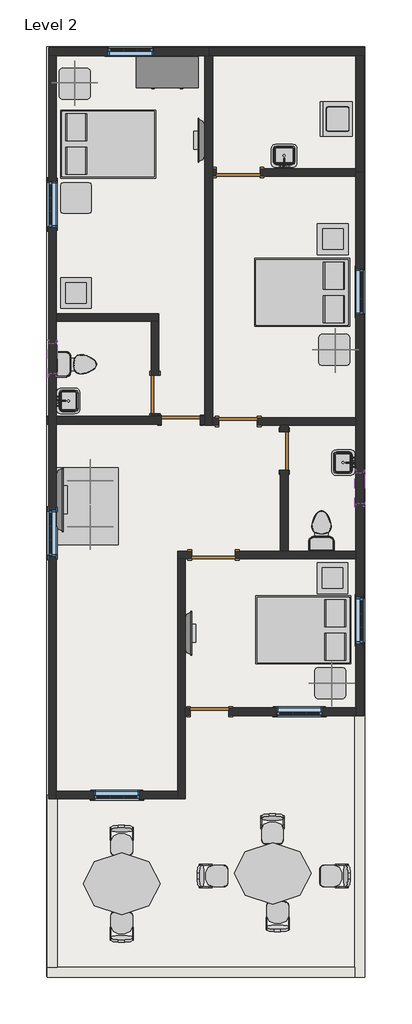
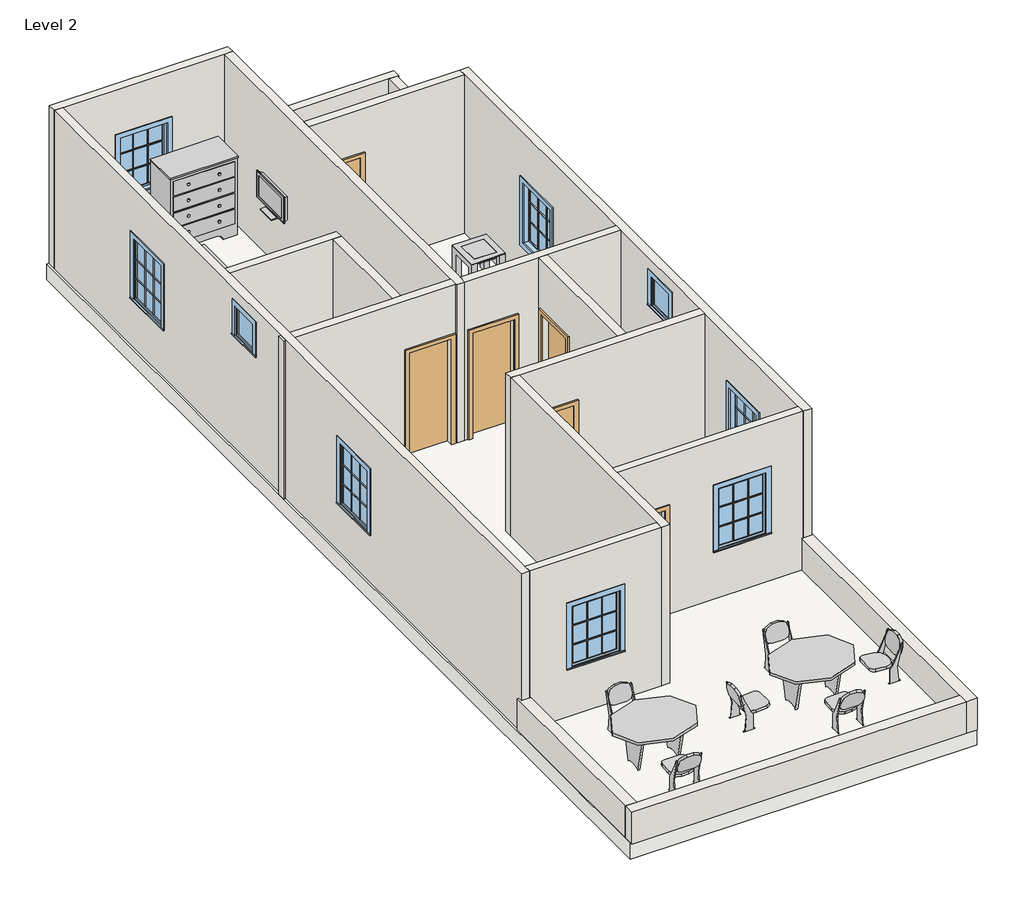
# One storey, incomplete: 23 furniture elements, 19 walls, 9 windows, 7 doors, 7 flow terminals, 5 geographic elements, 1 proxy, 1 slab.
"""IFC4 building model written with IfcOpenShell, lengths in millimetres."""

from ifc_helpers import new_model, si_unit, frame, origin, place, context, project, spatial, polyline, outline, extrude, faceted_brep, transform, mapped, element, save
from components import proxy_718fa39f, door_255cab33, door_059fdd7e, door_b6e9fca3, flow_terminal_accce45a, flow_terminal_62a433f7, toilet_domestic_3d_toilet_domestic_3d_f7549cf7, toilet_domestic_3d_toilet_domestic_3d_183bbd19, furniture_c8abb964, furniture_2babcf72, furniture_3d1d9cbc, furniture_56245f3a, furniture_fdf74506, furniture_b5c51a22, furniture_743965d2, furniture_31d08a24, furniture_e8434c74, rpc_plant_tropical_agave_1_5_93a2a214, window_5c190c7e, window_3d781103

model = new_model("IFC4")

# Units and contexts
model_context = context("Model", 3, world=origin())
ifc_project = project(units=[si_unit("LENGTHUNIT", "METRE", prefix="MILLI")], contexts=[model_context])

# Site, building, storey
site = spatial("IfcSite", under=ifc_project)
building = spatial("IfcBuilding", under=site)
storey = spatial("IfcBuildingStorey", under=building, Name="Level 2", Elevation=3048.0)

# Proxy
placement = place(None, origin())
proxy_shape = proxy_718fa39f(model_context)
element("IfcBuildingElementProxy", 1, Name="Washer : 27\" x 25\" x 35\"", ObjectType="Washer : 27\" x 25\" x 35\"", at=placement, inside=storey, context=model_context, shape_type="MappedRepresentation", body=[
    mapped(proxy_shape, transform((2989.1016011, 11111.8929316, 3048.0), x_axis=(0.0, 1.0000000000000007, 0.0), y_axis=(-1.0000000000000007, 0.0, 0.0), z_axis=(0.0, 0.0, 1.0))),
])

# Doors
door_shape = door_255cab33(model_context)
element("IfcDoor", 2, ObjectType="Single-Flush : 30\" x 80\"", at=placement, inside=storey, context=model_context, shape_type="MappedRepresentation", body=[
    mapped(door_shape, transform((-870.8676675, 6084.0104001, 3048.0), x_axis=(0.0, -1.0, 0.0), y_axis=(1.0, 0.0, 0.0), z_axis=(0.0, 0.0, 1.0))),
])
element("IfcDoor", 3, ObjectType="Single-Flush : 30\" x 80\"", at=placement, inside=storey, context=model_context, shape_type="MappedRepresentation", body=[
    mapped(door_shape, transform((773.4921844, 5550.6104001, 3048.0), x_axis=(-1.0, 0.0, 0.0), y_axis=(0.0, -1.0, 0.0), z_axis=(0.0, 0.0, 1.0))),
])
element("IfcDoor", 4, ObjectType="Single-Flush : 30\" x 80\"", at=placement, inside=storey, context=model_context, shape_type="MappedRepresentation", body=[
    mapped(door_shape, transform((1684.5721104, 4966.4104001, 3048.0), x_axis=(0.0, 1.0, 0.0), y_axis=(-1.0, 0.0, 0.0), z_axis=(0.0, 0.0, 1.0))),
])
element("IfcDoor", 5, ObjectType="Single-Flush : 30\" x 80\"", at=placement, inside=storey, context=model_context, shape_type="MappedRepresentation", body=[
    mapped(door_shape, transform((208.0520363, -189.7895999, 3048.0), x_axis=(-1.0, 0.0, 0.0), y_axis=(0.0, -1.0, 0.0), z_axis=(0.0, 0.0, 1.0))),
])
door_2_shape = door_059fdd7e(model_context)
element("IfcDoor", 6, ObjectType="Single-Flush : 30\" x 80\"", at=placement, inside=storey, context=model_context, shape_type="MappedRepresentation", body=[
    mapped(door_2_shape, transform((-362.8676675, 5576.0104001, 3048.0), x_axis=(1.0, 0.0, 0.0), y_axis=(0.0, 1.0, 0.0), z_axis=(0.0, 0.0, 1.0))),
])
door_3_shape = door_b6e9fca3(model_context)
element("IfcDoor", 7, ObjectType="Single-Flush : 34\" x 84\"", at=placement, inside=storey, context=model_context, shape_type="MappedRepresentation", body=[
    mapped(door_3_shape, transform((773.4921844, 10478.2104001, 3048.0), x_axis=(-1.0, 0.0, 0.0), y_axis=(0.0, -1.0, 0.0), z_axis=(0.0, 0.0, 1.0))),
])
element("IfcDoor", 8, ObjectType="Single-Flush : 34\" x 84\"", at=placement, inside=storey, context=model_context, shape_type="MappedRepresentation", body=[
    mapped(door_3_shape, transform((284.2520363, 2909.0104001, 3048.0), x_axis=(-1.0, 0.0, 0.0), y_axis=(0.0, -1.0, 0.0), z_axis=(0.0, 0.0, 1.0))),
])

# Flow terminals
flow_terminal_shape = flow_terminal_accce45a(model_context)
element("IfcFlowTerminal", 9, ObjectType="Floor Drain - Round : 5\" Strainer - 2\" Drain", at=placement, inside=storey, context=model_context, shape_type="MappedRepresentation", body=[
    mapped(flow_terminal_shape, transform((2849.6520363, 3798.0104001, 3048.0), x_axis=(1.0, 0.0, 0.0), y_axis=(0.0, 1.0, 0.0), z_axis=(0.0, 0.0, 1.0))),
])
element("IfcFlowTerminal", 10, ObjectType="Floor Drain - Round : 5\" Strainer - 2\" Drain", at=placement, inside=storey, context=model_context, shape_type="MappedRepresentation", body=[
    mapped(flow_terminal_shape, transform((-2331.9479637, 7125.4104001, 3048.0), x_axis=(1.0, 0.0, 0.0), y_axis=(0.0, 1.0, 0.0), z_axis=(0.0, 0.0, 1.0))),
])
flow_terminal_2_shape = flow_terminal_62a433f7(model_context)
element("IfcFlowTerminal", 11, ObjectType="Sink Vanity-Square : 20\" x 18\"", at=placement, inside=storey, context=model_context, shape_type="MappedRepresentation", body=[
    mapped(flow_terminal_2_shape, transform((-2634.4025626, 5941.3211595, 3048.0), x_axis=(0.0, 1.0000000000000002, 0.0), y_axis=(-1.0000000000000002, 0.0, 0.0), z_axis=(0.0, 0.0, 1.0))),
])
element("IfcFlowTerminal", 12, ObjectType="Sink Vanity-Square : 20\" x 18\"", at=placement, inside=storey, context=model_context, shape_type="MappedRepresentation", body=[
    mapped(flow_terminal_2_shape, transform((2898.1066352, 4753.4996407, 3048.0), x_axis=(0.0, -1.0, 0.0), y_axis=(1.0, 0.0, 0.0), z_axis=(0.0, 0.0, 1.0))),
])
element("IfcFlowTerminal", 13, ObjectType="Sink Vanity-Square : 20\" x 18\"", at=placement, inside=storey, context=model_context, shape_type="MappedRepresentation", body=[
    mapped(flow_terminal_2_shape, transform((1696.9412769, 10759.9558012, 3048.0), x_axis=(-1.0000000000000004, 0.0, 0.0), y_axis=(0.0, -1.0000000000000004, 0.0), z_axis=(0.0, 0.0, 1.0))),
])
toilet_domestic_3d_toilet_domestic_3d_shape = toilet_domestic_3d_toilet_domestic_3d_f7549cf7(model_context)
toilet_domestic_3d_toilet_domestic_3d_2_shape = toilet_domestic_3d_toilet_domestic_3d_183bbd19(model_context)
element("IfcFlowTerminal", 14, ObjectType="Toilet-Domestic-3D : Toilet-Domestic-3D", at=placement, inside=storey, context=model_context, shape_type="MappedRepresentation", body=[
    mapped(toilet_domestic_3d_toilet_domestic_3d_shape, transform((-2331.9716402, 6680.9104001, 3048.0), x_axis=(0.0, 1.0000000000000002, 0.0), y_axis=(-1.0000000000000002, 0.0, 0.0), z_axis=(0.0, 0.0, 1.0))),
    mapped(toilet_domestic_3d_toilet_domestic_3d_2_shape, transform((-2331.9716402, 6680.9104001, 3048.0), x_axis=(0.0, 1.0000000000000002, 0.0), y_axis=(-1.0000000000000002, 0.0, 0.0), z_axis=(0.0, 0.0, 1.0))),
])
element("IfcFlowTerminal", 15, ObjectType="Toilet-Domestic-3D : Toilet-Domestic-3D", at=placement, inside=storey, context=model_context, shape_type="MappedRepresentation", body=[
    mapped(toilet_domestic_3d_toilet_domestic_3d_shape, transform((2421.1721104, 3479.9064275, 3048.0), x_axis=(-1.0000000000000004, 0.0, 0.0), y_axis=(0.0, -1.0000000000000004, 0.0), z_axis=(0.0, 0.0, 1.0))),
    mapped(toilet_domestic_3d_toilet_domestic_3d_2_shape, transform((2421.1721104, 3479.9064275, 3048.0), x_axis=(-1.0000000000000004, 0.0, 0.0), y_axis=(0.0, -1.0000000000000004, 0.0), z_axis=(0.0, 0.0, 1.0))),
])

# Furniture
furniture_shape = furniture_c8abb964(model_context)
element("IfcFurniture", 16, ObjectType="Bed-Box : Double 53\" x 74\"", at=placement, inside=storey, context=model_context, shape_type="MappedRepresentation", body=[
    mapped(furniture_shape, transform((-2032.9774719, 10697.8579411, 3048.0), x_axis=(0.0, 1.0, 0.0), y_axis=(-1.0, 0.0, 0.0), z_axis=(0.0, 0.0, 1.0))),
])
element("IfcFurniture", 17, ObjectType="Bed-Box : Double 53\" x 74\"", at=placement, inside=storey, context=model_context, shape_type="MappedRepresentation", body=[
    mapped(furniture_shape, transform((2271.2815445, 8442.4628591, 3048.0), x_axis=(0.0, -1.0, 0.0), y_axis=(1.0, 0.0, 0.0), z_axis=(0.0, 0.0, 1.0))),
])
element("IfcFurniture", 18, ObjectType="Bed-Box : Double 53\" x 74\"", at=placement, inside=storey, context=model_context, shape_type="MappedRepresentation", body=[
    mapped(furniture_shape, transform((2296.6815445, 1765.7892779, 3048.0), x_axis=(0.0, -1.0000000000000002, 0.0), y_axis=(1.0000000000000002, 0.0, 0.0), z_axis=(0.0, 0.0, 1.0))),
])
furniture_2_shape = furniture_2babcf72(model_context)
element("IfcFurniture", 19, ObjectType="Dresser : 48\" x 60\" x 24\"", at=placement, inside=storey, context=model_context, shape_type="MappedRepresentation", body=[
    mapped(furniture_2_shape, transform((-360.9547039, 12822.5733542, 3048.0), x_axis=(1.0, 0.0, 0.0), y_axis=(0.0, 1.0, 0.0), z_axis=(0.0, 0.0, 1.0))),
])
furniture_3_shape = furniture_3d1d9cbc(model_context)
element("IfcFurniture", 20, ObjectType="Seating-Auditorium : 18\" x 24\" x 30\"", at=placement, inside=storey, context=model_context, shape_type="MappedRepresentation", body=[
    mapped(furniture_3_shape, transform((-1371.1200948, -2539.9141901, 3048.0), x_axis=(-1.0000000000000004, 0.0, 0.0), y_axis=(0.0, -1.0000000000000004, 0.0), z_axis=(0.0, 0.0, 1.0))),
])
element("IfcFurniture", 21, ObjectType="Seating-Auditorium : 18\" x 24\" x 30\"", at=placement, inside=storey, context=model_context, shape_type="MappedRepresentation", body=[
    mapped(furniture_3_shape, transform((1613.3799052, -2311.3141901, 3048.0), x_axis=(-1.0000000000000004, 0.0, 0.0), y_axis=(0.0, -1.0000000000000004, 0.0), z_axis=(0.0, 0.0, 1.0))),
])
element("IfcFurniture", 22, ObjectType="Seating-Auditorium : 18\" x 24\" x 30\"", at=placement, inside=storey, context=model_context, shape_type="MappedRepresentation", body=[
    mapped(furniture_3_shape, transform((1393.5241675, -4443.6650097, 3048.0), x_axis=(1.0, 0.0, 0.0), y_axis=(0.0, 1.0, 0.0), z_axis=(0.0, 0.0, 1.0))),
])
element("IfcFurniture", 23, ObjectType="Seating-Auditorium : 18\" x 24\" x 30\"", at=placement, inside=storey, context=model_context, shape_type="MappedRepresentation", body=[
    mapped(furniture_3_shape, transform((68.9766265, -3280.261731, 3048.0), x_axis=(0.0, -1.0000000000000007, 0.0), y_axis=(1.0000000000000007, 0.0, 0.0), z_axis=(0.0, 0.0, 1.0))),
])
element("IfcFurniture", 24, ObjectType="Seating-Auditorium : 18\" x 24\" x 30\"", at=placement, inside=storey, context=model_context, shape_type="MappedRepresentation", body=[
    mapped(furniture_3_shape, transform((2887.1274461, -3601.7174688, 3048.0), x_axis=(0.0, 1.000000000000001, 0.0), y_axis=(-1.000000000000001, 0.0, 0.0), z_axis=(0.0, 0.0, 1.0))),
])
element("IfcFurniture", 25, ObjectType="Seating-Auditorium : 18\" x 24\" x 30\"", at=placement, inside=storey, context=model_context, shape_type="MappedRepresentation", body=[
    mapped(furniture_3_shape, transform((-1692.5758325, -4646.8650097, 3048.0), x_axis=(1.0, 0.0, 0.0), y_axis=(0.0, 1.0, 0.0), z_axis=(0.0, 0.0, 1.0))),
])
furniture_4_shape = furniture_56245f3a(model_context)
element("IfcFurniture", 26, ObjectType="TV - Flat Screen : 32\"", at=placement, inside=storey, context=model_context, shape_type="MappedRepresentation", body=[
    mapped(furniture_4_shape, transform((47.9134127, 11109.265886, 4089.4), x_axis=(0.0, -1.0000000000000002, 0.0), y_axis=(1.0000000000000002, 0.0, 0.0), z_axis=(0.0, 0.0, 1.0))),
])
element("IfcFurniture", 27, ObjectType="TV - Flat Screen : 32\"", at=placement, inside=storey, context=model_context, shape_type="MappedRepresentation", body=[
    mapped(furniture_4_shape, transform((-216.00934, 1363.5549142, 3962.4), x_axis=(0.0, 1.0000000000000002, 0.0), y_axis=(-1.0000000000000002, 0.0, 0.0), z_axis=(0.0, 0.0, 1.0))),
])
furniture_5_shape = furniture_fdf74506(model_context)
element("IfcFurniture", 28, ObjectType="TV - Flat Screen : 50\"", at=placement, inside=storey, context=model_context, shape_type="MappedRepresentation", body=[
    mapped(furniture_5_shape, transform((-2756.00934, 4005.1549142, 4089.4), x_axis=(0.0, 1.0000000000000002, 0.0), y_axis=(-1.0000000000000002, 0.0, 0.0), z_axis=(0.0, 0.0, 1.0))),
])
furniture_6_shape = furniture_b5c51a22(model_context)
element("IfcFurniture", 29, ObjectType="Table-Coffee : 24\" x 24\" x 24\"", at=placement, inside=storey, context=model_context, shape_type="MappedRepresentation", body=[
    mapped(furniture_6_shape, transform((-2451.8137304, 7995.3993223, 3048.0), x_axis=(1.0, 0.0, 0.0), y_axis=(0.0, 1.0, 0.0), z_axis=(0.0, 0.0, 1.0))),
])
element("IfcFurniture", 30, ObjectType="Table-Coffee : 24\" x 24\" x 24\"", at=placement, inside=storey, context=model_context, shape_type="MappedRepresentation", body=[
    mapped(furniture_6_shape, transform((2628.1862696, 9062.1993223, 3048.0), x_axis=(1.0, 0.0, 0.0), y_axis=(0.0, 1.0, 0.0), z_axis=(0.0, 0.0, 1.0))),
])
element("IfcFurniture", 31, ObjectType="Table-Coffee : 24\" x 24\" x 24\"", at=placement, inside=storey, context=model_context, shape_type="MappedRepresentation", body=[
    mapped(furniture_6_shape, transform((2621.8362696, 2356.5993223, 3048.0), x_axis=(1.0, 0.0, 0.0), y_axis=(0.0, 1.0, 0.0), z_axis=(0.0, 0.0, 1.0))),
])
furniture_7_shape = furniture_743965d2(model_context)
element("IfcFurniture", 32, ObjectType="Table-Ellipse : 60\" x 48\"", at=placement, inside=storey, context=model_context, shape_type="MappedRepresentation", body=[
    mapped(furniture_7_shape, transform((-1531.8479637, -3593.3895999, 3048.0), x_axis=(1.0, 0.0, 0.0), y_axis=(0.0, 1.0, 0.0), z_axis=(0.0, 0.0, 1.0))),
])
element("IfcFurniture", 33, ObjectType="Table-Ellipse : 60\" x 48\"", at=placement, inside=storey, context=model_context, shape_type="MappedRepresentation", body=[
    mapped(furniture_7_shape, transform((1452.6520363, -3390.1895999, 3048.0), x_axis=(1.0, 0.0, 0.0), y_axis=(0.0, 1.0, 0.0), z_axis=(0.0, 0.0, 1.0))),
])
furniture_8_shape = furniture_31d08a24(model_context)
element("IfcFurniture", 34, ObjectType="Table-End : 24\" x 24\"", at=placement, inside=storey, context=model_context, shape_type="MappedRepresentation", body=[
    mapped(furniture_8_shape, transform((-2767.481594, 12078.4104001, 3048.0), x_axis=(1.0, 0.0, 0.0), y_axis=(0.0, 1.0, 0.0), z_axis=(0.0, 0.0, 1.0))),
])
element("IfcFurniture", 35, ObjectType="Table-End : 24\" x 24\"", at=placement, inside=storey, context=model_context, shape_type="MappedRepresentation", body=[
    mapped(furniture_8_shape, transform((-2742.081594, 9817.8104001, 3048.0), x_axis=(1.0, 0.0, 0.0), y_axis=(0.0, 1.0, 0.0), z_axis=(0.0, 0.0, 1.0))),
])
element("IfcFurniture", 36, ObjectType="Table-End : 24\" x 24\"", at=placement, inside=storey, context=model_context, shape_type="MappedRepresentation", body=[
    mapped(furniture_8_shape, transform((2363.318406, 6814.2604001, 3048.0), x_axis=(1.0, 0.0, 0.0), y_axis=(0.0, 1.0, 0.0), z_axis=(0.0, 0.0, 1.0))),
])
element("IfcFurniture", 37, ObjectType="Table-End : 24\" x 24\"", at=placement, inside=storey, context=model_context, shape_type="MappedRepresentation", body=[
    mapped(furniture_8_shape, transform((2287.118406, 222.9604001, 3048.0), x_axis=(1.0, 0.0, 0.0), y_axis=(0.0, 1.0, 0.0), z_axis=(0.0, 0.0, 1.0))),
])
furniture_9_shape = furniture_e8434c74(model_context)
element("IfcFurniture", 38, ObjectType="Table-Rectangular : 60\" x 48\"", at=placement, inside=storey, context=model_context, shape_type="MappedRepresentation", body=[
    mapped(furniture_9_shape, transform((-2204.9479637, 3874.2104001, 3048.0), x_axis=(0.0, 1.0, 0.0), y_axis=(-1.0, 0.0, 0.0), z_axis=(0.0, 0.0, 1.0))),
])

# Geographic elements
rpc_plant_tropical_agave_1_5_shape = rpc_plant_tropical_agave_1_5_93a2a214(model_context)
element("IfcGeographicElement", 39, ObjectType="RPC Plant - Tropical : Agave - 1.5'", at=placement, inside=storey, context=model_context, shape_type="MappedRepresentation", body=[
    mapped(rpc_plant_tropical_agave_1_5_shape, transform((-2458.9479637, 12256.2104001, 3657.6), x_axis=(1.0, 0.0, 0.0), y_axis=(0.0, 1.0, 0.0), z_axis=(0.0, 0.0, 1.0))),
])
element("IfcGeographicElement", 40, ObjectType="RPC Plant - Tropical : Agave - 1.5'", at=placement, inside=storey, context=model_context, shape_type="MappedRepresentation", body=[
    mapped(rpc_plant_tropical_agave_1_5_shape, transform((2697.2520363, 6966.6604001, 3657.6), x_axis=(1.0, 0.0, 0.0), y_axis=(0.0, 1.0, 0.0), z_axis=(0.0, 0.0, 1.0))),
])
element("IfcGeographicElement", 41, ObjectType="RPC Plant - Tropical : Agave - 1.5'", at=placement, inside=storey, context=model_context, shape_type="MappedRepresentation", body=[
    mapped(rpc_plant_tropical_agave_1_5_shape, transform((2621.0520363, 375.3604001, 3657.6), x_axis=(1.0, 0.0, 0.0), y_axis=(0.0, 1.0, 0.0), z_axis=(0.0, 0.0, 1.0))),
])
element("IfcGeographicElement", 42, ObjectType="RPC Plant - Tropical : Agave - 1.5'", at=placement, inside=storey, context=model_context, shape_type="MappedRepresentation", body=[
    mapped(rpc_plant_tropical_agave_1_5_shape, transform((-2154.1479637, 4382.2104001, 3708.4), x_axis=(1.0, 0.0, 0.0), y_axis=(0.0, 1.0, 0.0), z_axis=(0.0, 0.0, 1.0))),
])
element("IfcGeographicElement", 43, ObjectType="RPC Plant - Tropical : Agave - 1.5'", at=placement, inside=storey, context=model_context, shape_type="MappedRepresentation", body=[
    mapped(rpc_plant_tropical_agave_1_5_shape, transform((-2154.1479637, 3467.8104001, 3708.4), x_axis=(1.0, 0.0, 0.0), y_axis=(0.0, 1.0, 0.0), z_axis=(0.0, 0.0, 1.0))),
])

# Slab
element("IfcSlab", 44, ObjectType="Generic - 12\" 2", at=placement, inside=storey, context=model_context, shape_type="SweptSolid", body=[
    extrude(outline(polyline([(3281.4520363, 12967.4104001), (3281.4520363, -5422.1895999), (-3017.7479637, -5422.1895999), (-3017.7479637, 12967.4104001), (3281.4520363, 12967.4104001)])), frame((0.0, 0.0, 2743.2), z_axis=(0.0, 0.0, 1.0), x_axis=(1.0, 0.0, 0.0)), (0.0, 0.0, 1.0), 304.8),
])

# Walls
element("IfcWall", 45, ObjectType="Generic - 2'", at=placement, inside=storey, context=model_context, shape_type="Brep", body=[
    faceted_brep([(3078.2520363, -5244.3895999, 3048.0), (-2801.2676675, -5244.3895999, 3048.0), (-3004.4676675, -5244.3895999, 3048.0), (-3004.4676675, -5244.3895999, 3657.6), (-2801.2676675, -5244.3895999, 3657.6), (3078.2520363, -5244.3895999, 3657.6), (3078.2520363, -5447.5895999, 3048.0), (3078.2520363, -5447.5895999, 3657.6), (-3004.4676675, -5447.5895999, 3657.6), (-3004.4676675, -5447.5895999, 3048.0)], [[[0, 1, 2, 3, 4, 5]], [[6, 7, 8, 9]], [[2, 1, 0, 6, 9]], [[5, 4, 3, 8, 7]], [[0, 5, 7, 6]], [[3, 2, 9, 8]]]),
])
element("IfcWall", 46, ObjectType="Generic - 2'", at=placement, inside=storey, context=model_context, shape_type="Brep", body=[
    faceted_brep([(-2801.2676675, -5244.3895999, 3048.0), (-2801.2676675, -1916.9895999, 3048.0), (-2801.2676675, -1840.7895999, 3048.0), (-2801.2676675, -1840.7895999, 3657.6), (-2801.2676675, -1916.9895999, 3657.6), (-2801.2676675, -5244.3895999, 3657.6), (-3004.4676675, -5244.3895999, 3048.0), (-3004.4676675, -5244.3895999, 3657.6), (-3004.4676675, -1840.7895999, 3657.6), (-3004.4676675, -1840.7895999, 3048.0), (-2979.0676675, -1840.7895999, 3048.0), (-2826.6676675, -1840.7895999, 3048.0), (-2979.0676675, -1840.7895999, 3657.6), (-2826.6676675, -1840.7895999, 3657.6)], [[[0, 1, 2, 3, 4, 5]], [[6, 7, 8, 9]], [[2, 1, 0, 6, 9, 10, 11]], [[3, 2, 11, 10, 9, 8, 12, 13]], [[5, 4, 3, 13, 12, 8, 7]], [[0, 5, 7, 6]]]),
])
element("IfcWall", 47, ObjectType="Generic - 2'", at=placement, inside=storey, context=model_context, shape_type="Brep", body=[
    faceted_brep([(3078.2520363, -189.7895999, 3048.0), (3078.2520363, -265.9895999, 3048.0), (3078.2520363, -5244.3895999, 3048.0), (3078.2520363, -5447.5895999, 3048.0), (3078.2520363, -5447.5895999, 3657.6), (3078.2520363, -5244.3895999, 3657.6), (3078.2520363, -265.9895999, 3657.6), (3078.2520363, -189.7895999, 3657.6), (3281.4520363, -189.7895999, 3048.0), (3281.4520363, -189.7895999, 3657.6), (3281.4520363, -5447.5895999, 3657.6), (3281.4520363, -5447.5895999, 3048.0), (3103.6520363, -189.7895999, 3048.0), (3256.0520363, -189.7895999, 3048.0), (3256.0520363, -189.7895999, 3657.6), (3103.6520363, -189.7895999, 3657.6)], [[[0, 1, 2, 3, 4, 5, 6, 7]], [[8, 9, 10, 11]], [[3, 2, 1, 0, 12, 13, 8, 11]], [[7, 6, 5, 4, 10, 9, 14, 15]], [[0, 7, 15, 14, 9, 8, 13, 12]], [[4, 3, 11, 10]]]),
])
element("IfcWall", 48, ObjectType="Generic - 6'", at=placement, inside=storey, context=model_context, shape_type="Brep", body=[
    faceted_brep([(-2979.0676675, 12789.6104001, 3048.0), (-2826.6676675, 12789.6104001, 3048.0), (113.0921844, 12789.6104001, 3048.0), (189.2921844, 12789.6104001, 3048.0), (189.2921844, 12789.6104001, 4572.0), (265.4921844, 12789.6104001, 4572.0), (265.4921844, 12789.6104001, 6096.0), (113.0921844, 12789.6104001, 6096.0), (-2826.6676675, 12789.6104001, 6096.0), (-2979.0676675, 12789.6104001, 6096.0), (-899.5877416, 12789.6104001, 5181.6), (-899.5877416, 12789.6104001, 3962.4), (-1813.9877416, 12789.6104001, 3962.4), (-1813.9877416, 12789.6104001, 5181.6), (-2979.0676675, 12942.0104001, 3048.0), (-2979.0676675, 12942.0104001, 6096.0), (265.4921844, 12942.0104001, 6096.0), (265.4921844, 12942.0104001, 4572.0), (189.2921844, 12942.0104001, 4572.0), (189.2921844, 12942.0104001, 3048.0), (-899.5877416, 12942.0104001, 5181.6), (-1813.9877416, 12942.0104001, 5181.6), (-1813.9877416, 12942.0104001, 3962.4), (-899.5877416, 12942.0104001, 3962.4)], [[[0, 1, 2, 3, 4, 5, 6, 7, 8, 9], [10, 11, 12, 13]], [[14, 15, 16, 17, 18, 19], [20, 21, 22, 23]], [[3, 2, 1, 0, 14, 19]], [[9, 8, 7, 6, 16, 15]], [[0, 9, 15, 14]], [[11, 10, 20, 23]], [[12, 11, 23, 22]], [[13, 12, 22, 21]], [[10, 13, 21, 20]], [[4, 3, 19, 18]], [[17, 5, 4, 18]], [[6, 5, 17, 16]]]),
])
element("IfcWall", 49, ObjectType="Generic - 6'", at=placement, inside=storey, context=model_context, shape_type="Brep", body=[
    faceted_brep([(3103.6520363, 12789.6104001, 3048.0), (3103.6520363, 10554.4104001, 3048.0), (3103.6520363, 10478.2104001, 3048.0), (3103.6520363, 10478.2104001, 4572.0), (3103.6520363, 10554.4104001, 4572.0), (3103.6520363, 12789.6104001, 4572.0), (3256.0520363, 12789.6104001, 3048.0), (3256.0520363, 12789.6104001, 4572.0), (3256.0520363, 10554.4104001, 4572.0), (3256.0520363, 10478.2104001, 4572.0), (3256.0520363, 10478.2104001, 3048.0)], [[[0, 1, 2, 3, 4, 5]], [[6, 7, 8, 9, 10]], [[2, 1, 0, 6, 10]], [[3, 2, 10, 9]], [[5, 4, 3, 9, 8, 7]], [[0, 5, 7, 6]]]),
])
element("IfcWall", 50, ObjectType="Generic - 6'", at=placement, inside=storey, context=model_context, shape_type="Brep", body=[
    faceted_brep([(113.0921844, 12789.6104001, 6096.0), (113.0921844, 12789.6104001, 3048.0), (113.0921844, 5652.2104001, 3048.0), (113.0921844, 5499.8104001, 3048.0), (113.0921844, 5474.4104001, 3048.0), (113.0921844, 5474.4104001, 6096.0), (113.0921844, 5499.8104001, 6096.0), (113.0921844, 5652.2104001, 6096.0), (265.4921844, 12789.6104001, 3048.0), (265.4921844, 12789.6104001, 4572.0), (265.4921844, 12789.6104001, 6096.0), (265.4921844, 10554.4104001, 6096.0), (265.4921844, 10402.0104001, 6096.0), (265.4921844, 5626.8104001, 6096.0), (265.4921844, 5474.4104001, 6096.0), (265.4921844, 5474.4104001, 3048.0), (265.4921844, 5626.8104001, 3048.0), (265.4921844, 10402.0104001, 3048.0), (265.4921844, 10554.4104001, 3048.0), (189.2921844, 12789.6104001, 3048.0)], [[[0, 1, 2, 3, 4, 5, 6, 7]], [[8, 9, 10, 11, 12, 13, 14, 15, 16, 17, 18]], [[4, 3, 2, 1, 19, 8, 18, 17, 16, 15]], [[0, 7, 6, 5, 14, 13, 12, 11, 10]], [[5, 4, 15, 14]], [[0, 10, 9, 8, 19, 1]]]),
])
element("IfcWall", 51, ObjectType="Generic - 6'", at=placement, inside=storey, context=model_context, shape_type="Brep", body=[
    faceted_brep([(113.0921844, 5652.2104001, 3048.0), (18.1323325, 5652.2104001, 3048.0), (18.1323325, 5652.2104001, 5080.0), (-743.8676675, 5652.2104001, 5080.0), (-743.8676675, 5652.2104001, 3048.0), (-794.6676675, 5652.2104001, 3048.0), (-947.0676675, 5652.2104001, 3048.0), (-3017.7479637, 5652.2104001, 3048.0), (-3017.7479637, 5652.2104001, 6096.0), (-947.0676675, 5652.2104001, 6096.0), (-794.6676675, 5652.2104001, 6096.0), (113.0921844, 5652.2104001, 6096.0), (18.1323325, 5499.8104001, 5080.0), (18.1323325, 5499.8104001, 3048.0), (113.0921844, 5499.8104001, 3048.0), (113.0921844, 5499.8104001, 6096.0), (-3017.7479637, 5499.8104001, 6096.0), (-3017.7479637, 5499.8104001, 3048.0), (-743.8676675, 5499.8104001, 3048.0), (-743.8676675, 5499.8104001, 5080.0)], [[[0, 1, 2, 3, 4, 5, 6, 7, 8, 9, 10, 11]], [[12, 13, 14, 15, 16, 17, 18, 19]], [[18, 17, 7, 6, 5, 4]], [[14, 13, 1, 0]], [[8, 7, 17, 16]], [[11, 10, 9, 8, 16, 15]], [[0, 11, 15, 14]], [[2, 1, 13, 12]], [[3, 2, 12, 19]], [[4, 3, 19, 18]]]),
])
element("IfcWall", 52, ObjectType="Generic - 6'", at=placement, inside=storey, context=model_context, shape_type="Brep", body=[
    faceted_brep([(392.4921844, 5626.8104001, 5080.0), (392.4921844, 5626.8104001, 3048.0), (265.4921844, 5626.8104001, 3048.0), (265.4921844, 5626.8104001, 6096.0), (3103.6520363, 5626.8104001, 6096.0), (3103.6520363, 5626.8104001, 3048.0), (1154.4921844, 5626.8104001, 3048.0), (1154.4921844, 5626.8104001, 5080.0), (265.4921844, 5474.4104001, 3048.0), (392.4921844, 5474.4104001, 3048.0), (392.4921844, 5474.4104001, 5080.0), (1154.4921844, 5474.4104001, 5080.0), (1154.4921844, 5474.4104001, 3048.0), (1608.3721104, 5474.4104001, 3048.0), (1760.7721104, 5474.4104001, 3048.0), (3103.6520363, 5474.4104001, 3048.0), (3103.6520363, 5474.4104001, 6096.0), (1760.7721104, 5474.4104001, 6096.0), (1608.3721104, 5474.4104001, 6096.0), (265.4921844, 5474.4104001, 6096.0)], [[[0, 1, 2, 3, 4, 5, 6, 7]], [[8, 9, 10, 11, 12, 13, 14, 15, 16, 17, 18, 19]], [[6, 5, 15, 14, 13, 12]], [[2, 1, 9, 8]], [[4, 3, 19, 18, 17, 16]], [[5, 4, 16, 15]], [[3, 2, 8, 19]], [[10, 9, 1, 0]], [[11, 10, 0, 7]], [[12, 11, 7, 6]]]),
])
element("IfcWall", 53, ObjectType="Generic - 6'", at=placement, inside=storey, context=model_context, shape_type="Brep", body=[
    faceted_brep([(265.4921844, 10402.0104001, 3048.0), (341.6921844, 10402.0104001, 3048.0), (341.6921844, 10402.0104001, 5181.6), (1205.2921844, 10402.0104001, 5181.6), (1205.2921844, 10402.0104001, 3048.0), (3103.6520363, 10402.0104001, 3048.0), (3103.6520363, 10402.0104001, 6096.0), (265.4921844, 10402.0104001, 6096.0), (341.6921844, 10554.4104001, 5181.6), (341.6921844, 10554.4104001, 3048.0), (265.4921844, 10554.4104001, 3048.0), (265.4921844, 10554.4104001, 6096.0), (3103.6520363, 10554.4104001, 6096.0), (3103.6520363, 10554.4104001, 4572.0), (3103.6520363, 10554.4104001, 3048.0), (1205.2921844, 10554.4104001, 3048.0), (1205.2921844, 10554.4104001, 5181.6), (3103.6520363, 10478.2104001, 3048.0)], [[[0, 1, 2, 3, 4, 5, 6, 7]], [[8, 9, 10, 11, 12, 13, 14, 15, 16]], [[15, 14, 17, 5, 4]], [[10, 9, 1, 0]], [[7, 6, 12, 11]], [[0, 7, 11, 10]], [[2, 1, 9, 8]], [[3, 2, 8, 16]], [[4, 3, 16, 15]], [[5, 17, 14, 13, 12, 6]]]),
])
element("IfcWall", 54, ObjectType="Generic - 6'", at=placement, inside=storey, context=model_context, shape_type="Brep", body=[
    faceted_brep([(-2826.6676675, 7531.8104001, 3048.0), (-947.0676675, 7531.8104001, 3048.0), (-794.6676675, 7531.8104001, 3048.0), (-794.6676675, 7531.8104001, 6096.0), (-947.0676675, 7531.8104001, 6096.0), (-2826.6676675, 7531.8104001, 6096.0), (-2826.6676675, 7684.2104001, 3048.0), (-2826.6676675, 7684.2104001, 6096.0), (-794.6676675, 7684.2104001, 6096.0), (-794.6676675, 7684.2104001, 3048.0)], [[[0, 1, 2, 3, 4, 5]], [[6, 7, 8, 9]], [[2, 1, 0, 6, 9]], [[5, 4, 3, 8, 7]], [[0, 5, 7, 6]], [[3, 2, 9, 8]]]),
])
element("IfcWall", 55, ObjectType="Generic - 6'", at=placement, inside=storey, context=model_context, shape_type="SweptSolid", body=[
    extrude(outline(polyline([(5703.0104001, 5080.0), (5703.0104001, 3048.0), (5652.2104001, 3048.0), (5652.2104001, 6096.0), (7531.8104001, 6096.0), (7531.8104001, 3048.0), (6465.0104001, 3048.0), (6465.0104001, 5080.0), (5703.0104001, 5080.0)])), frame((-947.0676675, 0.0, 0.0), z_axis=(1.0, 0.0, 0.0), x_axis=(0.0, 1.0, 0.0)), (0.0, 0.0, 1.0), 152.4),
])
element("IfcWall", 56, ObjectType="Generic - 6'", at=placement, inside=storey, context=model_context, shape_type="SweptSolid", body=[
    extrude(outline(polyline([(5474.4104001, 3048.0), (5347.4104001, 3048.0), (5347.4104001, 5080.0), (4585.4104001, 5080.0), (4585.4104001, 3048.0), (2985.2104001, 3048.0), (2985.2104001, 6096.0), (5474.4104001, 6096.0), (5474.4104001, 3048.0)])), frame((1608.3721104, 0.0, 0.0), z_axis=(1.0, 0.0, 0.0), x_axis=(0.0, 1.0, 0.0)), (0.0, 0.0, 1.0), 152.4),
])
element("IfcWall", 57, ObjectType="Generic - 6'", at=placement, inside=storey, context=model_context, shape_type="Brep", body=[
    faceted_brep([(-426.9479637, 2832.8104001, 3048.0), (-274.5479637, 2832.8104001, 3048.0), (-147.5479637, 2832.8104001, 3048.0), (-147.5479637, 2832.8104001, 5181.6), (716.0520363, 2832.8104001, 5181.6), (716.0520363, 2832.8104001, 3048.0), (3103.6520363, 2832.8104001, 3048.0), (3103.6520363, 2832.8104001, 6096.0), (-274.5479637, 2832.8104001, 6096.0), (-426.9479637, 2832.8104001, 6096.0), (-147.5479637, 2985.2104001, 5181.6), (-147.5479637, 2985.2104001, 3048.0), (-426.9479637, 2985.2104001, 3048.0), (-426.9479637, 2985.2104001, 6096.0), (1608.3721104, 2985.2104001, 6096.0), (1760.7721104, 2985.2104001, 6096.0), (3103.6520363, 2985.2104001, 6096.0), (3103.6520363, 2985.2104001, 3048.0), (1760.7721104, 2985.2104001, 3048.0), (1608.3721104, 2985.2104001, 3048.0), (716.0520363, 2985.2104001, 3048.0), (716.0520363, 2985.2104001, 5181.6)], [[[0, 1, 2, 3, 4, 5, 6, 7, 8, 9]], [[10, 11, 12, 13, 14, 15, 16, 17, 18, 19, 20, 21]], [[12, 11, 2, 1, 0]], [[20, 19, 18, 17, 6, 5]], [[9, 8, 7, 16, 15, 14, 13]], [[7, 6, 17, 16]], [[0, 9, 13, 12]], [[3, 2, 11, 10]], [[4, 3, 10, 21]], [[5, 4, 21, 20]]]),
])
element("IfcWall", 58, ObjectType="Generic - 6'", at=placement, inside=storey, context=model_context, shape_type="Brep", body=[
    faceted_brep([(-426.9479637, 2832.8104001, 3048.0), (-426.9479637, -1764.5895999, 3048.0), (-426.9479637, -1916.9895999, 3048.0), (-426.9479637, -1916.9895999, 6096.0), (-426.9479637, -1764.5895999, 6096.0), (-426.9479637, 2832.8104001, 6096.0), (-274.5479637, 2832.8104001, 3048.0), (-274.5479637, 2832.8104001, 6096.0), (-274.5479637, -113.5895999, 6096.0), (-274.5479637, -265.9895999, 6096.0), (-274.5479637, -1916.9895999, 6096.0), (-274.5479637, -1916.9895999, 3048.0), (-274.5479637, -265.9895999, 3048.0), (-274.5479637, -113.5895999, 3048.0)], [[[0, 1, 2, 3, 4, 5]], [[6, 7, 8, 9, 10, 11, 12, 13]], [[2, 1, 0, 6, 13, 12, 11]], [[5, 4, 3, 10, 9, 8, 7]], [[0, 5, 7, 6]], [[3, 2, 11, 10]]]),
])
element("IfcWall", 59, ObjectType="Generic - 6'", at=placement, inside=storey, context=model_context, shape_type="Brep", body=[
    faceted_brep([(-274.5479637, -265.9895999, 3048.0), (-172.9479637, -265.9895999, 3048.0), (-172.9479637, -265.9895999, 5080.0), (589.0520363, -265.9895999, 5080.0), (589.0520363, -265.9895999, 3048.0), (3078.2520363, -265.9895999, 3048.0), (3078.2520363, -265.9895999, 3657.6), (3103.6520363, -265.9895999, 3657.6), (3103.6520363, -265.9895999, 6096.0), (-274.5479637, -265.9895999, 6096.0), (1528.8520363, -265.9895999, 5181.6), (2443.2520363, -265.9895999, 5181.6), (2443.2520363, -265.9895999, 3962.4), (1528.8520363, -265.9895999, 3962.4), (-172.9479637, -113.5895999, 5080.0), (-172.9479637, -113.5895999, 3048.0), (-274.5479637, -113.5895999, 3048.0), (-274.5479637, -113.5895999, 6096.0), (3103.6520363, -113.5895999, 6096.0), (3103.6520363, -113.5895999, 3657.6), (3103.6520363, -113.5895999, 3048.0), (589.0520363, -113.5895999, 3048.0), (589.0520363, -113.5895999, 5080.0), (1528.8520363, -113.5895999, 5181.6), (1528.8520363, -113.5895999, 3962.4), (2443.2520363, -113.5895999, 3962.4), (2443.2520363, -113.5895999, 5181.6), (3103.6520363, -189.7895999, 3048.0), (3078.2520363, -189.7895999, 3048.0), (3103.6520363, -189.7895999, 3657.6), (3078.2520363, -189.7895999, 3657.6)], [[[0, 1, 2, 3, 4, 5, 6, 7, 8, 9], [10, 11, 12, 13]], [[14, 15, 16, 17, 18, 19, 20, 21, 22], [23, 24, 25, 26]], [[21, 20, 27, 28, 5, 4]], [[16, 15, 1, 0]], [[9, 8, 18, 17]], [[0, 9, 17, 16]], [[29, 7, 6, 30]], [[6, 5, 28, 30]], [[8, 7, 29, 19, 18]], [[28, 27, 29, 30]], [[27, 20, 19, 29]], [[2, 1, 15, 14]], [[3, 2, 14, 22]], [[4, 3, 22, 21]], [[24, 23, 10, 13]], [[25, 24, 13, 12]], [[26, 25, 12, 11]], [[23, 26, 11, 10]]]),
])
element("IfcWall", 60, ObjectType="Generic - 6'", at=placement, inside=storey, context=model_context, shape_type="Brep", body=[
    faceted_brep([(-426.9479637, -1764.5895999, 3048.0), (-2826.6676675, -1764.5895999, 3048.0), (-2826.6676675, -1764.5895999, 3657.6), (-2826.6676675, -1764.5895999, 6096.0), (-426.9479637, -1764.5895999, 6096.0), (-2084.0078156, -1764.5895999, 5181.6), (-2084.0078156, -1764.5895999, 3962.4), (-1169.6078156, -1764.5895999, 3962.4), (-1169.6078156, -1764.5895999, 5181.6), (-426.9479637, -1916.9895999, 3048.0), (-426.9479637, -1916.9895999, 6096.0), (-2826.6676675, -1916.9895999, 6096.0), (-2826.6676675, -1916.9895999, 3657.6), (-2801.2676675, -1916.9895999, 3657.6), (-2801.2676675, -1916.9895999, 3048.0), (-2084.0078156, -1916.9895999, 5181.6), (-1169.6078156, -1916.9895999, 5181.6), (-1169.6078156, -1916.9895999, 3962.4), (-2084.0078156, -1916.9895999, 3962.4), (-2801.2676675, -1840.7895999, 3048.0), (-2826.6676675, -1840.7895999, 3048.0), (-2826.6676675, -1840.7895999, 3657.6), (-2801.2676675, -1840.7895999, 3657.6)], [[[0, 1, 2, 3, 4], [5, 6, 7, 8]], [[9, 10, 11, 12, 13, 14], [15, 16, 17, 18]], [[1, 0, 9, 14, 19, 20]], [[4, 3, 11, 10]], [[0, 4, 10, 9]], [[12, 21, 22, 13]], [[2, 1, 20, 21]], [[3, 2, 21, 12, 11]], [[20, 19, 22, 21]], [[19, 14, 13, 22]], [[6, 5, 15, 18]], [[7, 6, 18, 17]], [[8, 7, 17, 16]], [[5, 8, 16, 15]]]),
])
element("IfcWall", 61, ObjectType="Generic - 6'", at=placement, inside=storey, context=model_context, shape_type="Brep", body=[
    faceted_brep([(-2826.6676675, -1840.7895999, 3048.0), (-2826.6676675, -1764.5895999, 3048.0), (-2826.6676675, 7531.8104001, 3048.0), (-2826.6676675, 7684.2104001, 3048.0), (-2826.6676675, 12789.6104001, 3048.0), (-2826.6676675, 12789.6104001, 6096.0), (-2826.6676675, 7684.2104001, 6096.0), (-2826.6676675, 7531.8104001, 6096.0), (-2826.6676675, -1764.5895999, 6096.0), (-2826.6676675, -1916.9895999, 6096.0), (-2826.6676675, -1916.9895999, 3657.6), (-2826.6676675, -1840.7895999, 3657.6), (-2826.6676675, 10300.4104001, 5181.6), (-2826.6676675, 10300.4104001, 3962.4), (-2826.6676675, 9386.0104001, 3962.4), (-2826.6676675, 9386.0104001, 5181.6), (-2826.6676675, 3798.0104001, 5181.6), (-2826.6676675, 3798.0104001, 3962.4), (-2826.6676675, 2883.6104001, 3962.4), (-2826.6676675, 2883.6104001, 5181.6), (-2826.6676675, 7100.0104001, 5816.6), (-2826.6676675, 7100.0104001, 5207.0), (-2826.6676675, 6490.4104001, 5207.0), (-2826.6676675, 6490.4104001, 5816.6), (-2979.0676675, -1840.7895999, 3048.0), (-2979.0676675, -1840.7895999, 3657.6), (-2979.0676675, -1916.9895999, 3657.6), (-2979.0676675, -1916.9895999, 6096.0), (-2979.0676675, 12789.6104001, 6096.0), (-2979.0676675, 12789.6104001, 3048.0), (-2979.0676675, 10300.4104001, 5181.6), (-2979.0676675, 9386.0104001, 5181.6), (-2979.0676675, 9386.0104001, 3962.4), (-2979.0676675, 10300.4104001, 3962.4), (-2979.0676675, 3798.0104001, 5181.6), (-2979.0676675, 2883.6104001, 5181.6), (-2979.0676675, 2883.6104001, 3962.4), (-2979.0676675, 3798.0104001, 3962.4), (-2979.0676675, 7100.0104001, 5816.6), (-2979.0676675, 6490.4104001, 5816.6), (-2979.0676675, 6490.4104001, 5207.0), (-2979.0676675, 7100.0104001, 5207.0)], [[[0, 1, 2, 3, 4, 5, 6, 7, 8, 9, 10, 11], [12, 13, 14, 15], [16, 17, 18, 19], [20, 21, 22, 23]], [[24, 25, 26, 27, 28, 29], [30, 31, 32, 33], [34, 35, 36, 37], [38, 39, 40, 41]], [[4, 3, 2, 1, 0, 24, 29]], [[9, 8, 7, 6, 5, 28, 27]], [[5, 4, 29, 28]], [[0, 11, 25, 24]], [[10, 26, 25, 11]], [[10, 9, 27, 26]], [[13, 12, 30, 33]], [[14, 13, 33, 32]], [[15, 14, 32, 31]], [[12, 15, 31, 30]], [[17, 16, 34, 37]], [[18, 17, 37, 36]], [[19, 18, 36, 35]], [[16, 19, 35, 34]], [[21, 20, 38, 41]], [[22, 21, 41, 40]], [[23, 22, 40, 39]], [[20, 23, 39, 38]]]),
])
element("IfcWall", 62, ObjectType="Generic - 6'", at=placement, inside=storey, context=model_context, shape_type="Brep", body=[
    faceted_brep([(189.2921844, 12789.6104001, 3048.0), (265.4921844, 12789.6104001, 3048.0), (3103.6520363, 12789.6104001, 3048.0), (3256.0520363, 12789.6104001, 3048.0), (3281.4520363, 12789.6104001, 3048.0), (3281.4520363, 12789.6104001, 4572.0), (3256.0520363, 12789.6104001, 4572.0), (3103.6520363, 12789.6104001, 4572.0), (265.4921844, 12789.6104001, 4572.0), (189.2921844, 12789.6104001, 4572.0), (189.2921844, 12942.0104001, 3048.0), (189.2921844, 12942.0104001, 4572.0), (265.4921844, 12942.0104001, 4572.0), (3281.4520363, 12942.0104001, 4572.0), (3281.4520363, 12942.0104001, 3048.0)], [[[0, 1, 2, 3, 4, 5, 6, 7, 8, 9]], [[10, 11, 12, 13, 14]], [[4, 3, 2, 1, 0, 10, 14]], [[5, 4, 14, 13]], [[9, 8, 7, 6, 5, 13, 12, 11]], [[0, 9, 11, 10]]]),
])
element("IfcWall", 63, ObjectType="Generic - 6'", at=placement, inside=storey, context=model_context, shape_type="Brep", body=[
    faceted_brep([(3103.6520363, 10478.2104001, 3048.0), (3103.6520363, 10402.0104001, 3048.0), (3103.6520363, 5626.8104001, 3048.0), (3103.6520363, 5474.4104001, 3048.0), (3103.6520363, 2985.2104001, 3048.0), (3103.6520363, 2832.8104001, 3048.0), (3103.6520363, -113.5895999, 3048.0), (3103.6520363, -189.7895999, 3048.0), (3103.6520363, -189.7895999, 3657.6), (3103.6520363, -265.9895999, 3657.6), (3103.6520363, -265.9895999, 6096.0), (3103.6520363, -113.5895999, 6096.0), (3103.6520363, 2832.8104001, 6096.0), (3103.6520363, 2985.2104001, 6096.0), (3103.6520363, 5474.4104001, 6096.0), (3103.6520363, 5626.8104001, 6096.0), (3103.6520363, 10402.0104001, 6096.0), (3103.6520363, 10554.4104001, 6096.0), (3103.6520363, 10554.4104001, 4572.0), (3103.6520363, 10478.2104001, 4572.0), (3103.6520363, 7658.8104001, 5181.6), (3103.6520363, 7658.8104001, 3962.4), (3103.6520363, 8573.2104001, 3962.4), (3103.6520363, 8573.2104001, 5181.6), (3103.6520363, 1156.4104001, 5181.6), (3103.6520363, 1156.4104001, 3962.4), (3103.6520363, 2070.8104001, 3962.4), (3103.6520363, 2070.8104001, 5181.6), (3103.6520363, 4534.6104001, 5816.6), (3103.6520363, 3925.0104001, 5816.6), (3103.6520363, 3925.0104001, 5207.0), (3103.6520363, 4534.6104001, 5207.0), (3256.0520363, 10478.2104001, 3048.0), (3256.0520363, 10478.2104001, 4572.0), (3256.0520363, 10554.4104001, 4572.0), (3256.0520363, 10554.4104001, 6096.0), (3256.0520363, -265.9895999, 6096.0), (3256.0520363, -265.9895999, 3657.6), (3256.0520363, -189.7895999, 3657.6), (3256.0520363, -189.7895999, 3048.0), (3256.0520363, 7658.8104001, 5181.6), (3256.0520363, 8573.2104001, 5181.6), (3256.0520363, 8573.2104001, 3962.4), (3256.0520363, 7658.8104001, 3962.4), (3256.0520363, 1156.4104001, 5181.6), (3256.0520363, 2070.8104001, 5181.6), (3256.0520363, 2070.8104001, 3962.4), (3256.0520363, 1156.4104001, 3962.4), (3256.0520363, 4534.6104001, 5816.6), (3256.0520363, 4534.6104001, 5207.0), (3256.0520363, 3925.0104001, 5207.0), (3256.0520363, 3925.0104001, 5816.6)], [[[0, 1, 2, 3, 4, 5, 6, 7, 8, 9, 10, 11, 12, 13, 14, 15, 16, 17, 18, 19], [20, 21, 22, 23], [24, 25, 26, 27], [28, 29, 30, 31]], [[32, 33, 34, 35, 36, 37, 38, 39], [40, 41, 42, 43], [44, 45, 46, 47], [48, 49, 50, 51]], [[7, 6, 5, 4, 3, 2, 1, 0, 32, 39]], [[17, 16, 15, 14, 13, 12, 11, 10, 36, 35]], [[8, 7, 39, 38]], [[37, 9, 8, 38]], [[10, 9, 37, 36]], [[20, 23, 41, 40]], [[23, 22, 42, 41]], [[22, 21, 43, 42]], [[21, 20, 40, 43]], [[24, 27, 45, 44]], [[27, 26, 46, 45]], [[26, 25, 47, 46]], [[25, 24, 44, 47]], [[48, 51, 29, 28]], [[51, 50, 30, 29]], [[50, 49, 31, 30]], [[49, 48, 28, 31]], [[0, 19, 33, 32]], [[18, 34, 33, 19]], [[18, 17, 35, 34]]]),
])

# Windows
window_shape = window_5c190c7e(model_context)
element("IfcWindow", 64, ObjectType="Casement 3x3 with Trim : 36\" x 48\"", at=placement, inside=storey, context=model_context, shape_type="MappedRepresentation", body=[
    mapped(window_shape, transform((-1356.7877416, 12865.8104001, 3048.0), x_axis=(1.0, 0.0, 0.0), y_axis=(0.0, 1.0, 0.0), z_axis=(0.0, 0.0, 1.0))),
])
element("IfcWindow", 65, ObjectType="Casement 3x3 with Trim : 36\" x 48\"", at=placement, inside=storey, context=model_context, shape_type="MappedRepresentation", body=[
    mapped(window_shape, transform((-2902.8676675, 9843.2104001, 3048.0), x_axis=(0.0, 1.0, 0.0), y_axis=(-1.0, 0.0, 0.0), z_axis=(0.0, 0.0, 1.0))),
])
element("IfcWindow", 66, ObjectType="Casement 3x3 with Trim : 36\" x 48\"", at=placement, inside=storey, context=model_context, shape_type="MappedRepresentation", body=[
    mapped(window_shape, transform((3179.8520363, 8116.0104001, 3048.0), x_axis=(0.0, -1.0, 0.0), y_axis=(1.0, 0.0, 0.0), z_axis=(0.0, 0.0, 1.0))),
])
element("IfcWindow", 67, ObjectType="Casement 3x3 with Trim : 36\" x 48\"", at=placement, inside=storey, context=model_context, shape_type="MappedRepresentation", body=[
    mapped(window_shape, transform((-2902.8676675, 3340.8104001, 3048.0), x_axis=(0.0, 1.0, 0.0), y_axis=(-1.0, 0.0, 0.0), z_axis=(0.0, 0.0, 1.0))),
])
element("IfcWindow", 68, ObjectType="Casement 3x3 with Trim : 36\" x 48\"", at=placement, inside=storey, context=model_context, shape_type="MappedRepresentation", body=[
    mapped(window_shape, transform((-1626.8078156, -1840.7895999, 3048.0), x_axis=(-1.0, 0.0, 0.0), y_axis=(0.0, -1.0, 0.0), z_axis=(0.0, 0.0, 1.0))),
])
element("IfcWindow", 69, ObjectType="Casement 3x3 with Trim : 36\" x 48\"", at=placement, inside=storey, context=model_context, shape_type="MappedRepresentation", body=[
    mapped(window_shape, transform((1986.0520363, -189.7895999, 3048.0), x_axis=(-1.0, 0.0, 0.0), y_axis=(0.0, -1.0, 0.0), z_axis=(0.0, 0.0, 1.0))),
])
element("IfcWindow", 70, ObjectType="Casement 3x3 with Trim : 36\" x 48\"", at=placement, inside=storey, context=model_context, shape_type="MappedRepresentation", body=[
    mapped(window_shape, transform((3179.8520363, 1613.6104001, 3048.0), x_axis=(0.0, -1.0, 0.0), y_axis=(1.0, 0.0, 0.0), z_axis=(0.0, 0.0, 1.0))),
])
window_2_shape = window_3d781103(model_context)
element("IfcWindow", 71, ObjectType="Transom with Trim : 24\" x 24\"", at=placement, inside=storey, context=model_context, shape_type="MappedRepresentation", body=[
    mapped(window_2_shape, transform((3179.8520363, 4267.9104001, 3048.0), x_axis=(0.0, 1.0, 0.0), y_axis=(-1.0, 0.0, 0.0), z_axis=(0.0, 0.0, 1.0))),
])
element("IfcWindow", 72, ObjectType="Transom with Trim : 24\" x 24\"", at=placement, inside=storey, context=model_context, shape_type="MappedRepresentation", body=[
    mapped(window_2_shape, transform((-2902.8676675, 6833.3104001, 3048.0), x_axis=(0.0, 1.0, 0.0), y_axis=(-1.0, 0.0, 0.0), z_axis=(0.0, 0.0, 1.0))),
])

save(model, "model.ifc")

# Revit data of these elements
# Type "Washer : 27\" x 25\" x 35\""
#   Label = "W"
#   Assembly Code = "E1090400"
#   Depth = 2' - 1"
#   Height = 2' - 11"
#   Width = 2' - 3"
#   Washer Material = Steel, Paint Finish, Ivory, Matte
#   Default Elevation = 0
# Type "Single-Flush : 30\" x 80\""
#   Type Mark = "5"
#   Construction Type Id = "MDOOR"
#   Assembly Code = "C1020"
#   Analytic Construction = "Metal"
#   Thickness = 0' - 2"
#   Heat Transfer Coefficient (U) = 0.651978 BTU/(h·ft²·°F)
#   Height = 6' - 8"
#   Trim Projection Ext = 0' - 1"
#   Trim Projection Int = 0' - 1"
#   Trim Width = 0' - 3"
#   Width = 2' - 6"
#   Define Thermal Properties by = 1
#   Door Material = Door - Panel
#   Frame Material = Door - Frame
#   Visual Light Transmittance = 0
#   Solar Heat Gain Coefficient = 0
#   Function = (empty or 0)
#   Wall Closure = (empty or 0)
# Type "Single-Flush : 34\" x 84\""
#   Type Mark = "2"
#   Construction Type Id = "MDOOR"
#   Assembly Code = "C1020"
#   Analytic Construction = "Metal"
#   Thickness = 0' - 2"
#   Heat Transfer Coefficient (U) = 0.651978 BTU/(h·ft²·°F)
#   Height = 7' - 0"
#   Trim Projection Ext = 0' - 1"
#   Trim Projection Int = 0' - 1"
#   Trim Width = 0' - 3"
#   Width = 2' - 10"
#   Define Thermal Properties by = 1
#   Door Material = Door - Panel
#   Frame Material = Door - Frame
#   Visual Light Transmittance = 0
#   Solar Heat Gain Coefficient = 0
#   Function = (empty or 0)
#   Wall Closure = (empty or 0)
# Type "Floor Drain - Round : 5\" Strainer - 2\" Drain"
#   WFU = 2
#   Strainer Height = 0' - 3 1/4"
#   Strainer Radius = 0' - 2 1/2"
#   Strainer Diameter = 0' - 5"
#   Radius 6 = 0' - 0 5/8"
#   Radius 5 = 0' - 1 1/4"
#   Radius 4 = 0' - 1 7/8"
#   Radius 2 = 0' - 3.04167"
#   Radius 1 = 0' - 2.02083"
#   Radius 3 = 0' - 2 1/32"
#   Pipe Radius = 1"
#   Pipe Diameter = 2"
#   Height 2 = 0' - 0.725"
#   Height 1 = 0' - 1 13/16"
#   Body Radius = 0' - 4 1/16"
#   Body Height = 0' - 3 5/8"
#   Body Diameter = 0' - 8 1/8"
#   Drain Material = none
#   HWFU = 0
#   Default Elevation = 0
#   CWFU = 0
# Type "Sink Vanity-Square : 20\" x 18\""
#   Assembly Code = "D2010400"
#   Counter Height = 2' - 7"
#   Depth = 1' - 6"
#   Width = 1' - 8"
#   Basin Material = Porcelain, Linen
#   Faucet Material = Steel, Polished
#   Default Elevation = 0
# Type "Toilet-Domestic-3D : Toilet-Domestic-3D"
#   Assembly Code = "D2010110"
#   Toilet - Bowl/Basin Material = Porcelain, Linen
#   Toilet - Seat Material = Laminate, Linen, Matte
#   Default Elevation = 0
# Type "Bed-Box : Double 53\" x 74\""
#   Assembly Code = "E2020200"
#   Length = 6' - 2"
#   Width = 4' - 5"
#   Frame Material = Birch
#   Mattress Material = Linen, White
#   Default Elevation = 0
# Type "Dresser : 48\" x 60\" x 24\""
#   Assembly Code = "E2020200"
#   Depth = 2' - 0"
#   Height = 5' - 0"
#   Width = 4' - 0"
#   Dresser Material = Laminate - Ivory, Glossy
#   Drawer Material = Laminate, Ivory, Matte
#   Knob Material = Cherry
#   Default Elevation = 0
# Type "Seating-Auditorium : 18\" x 24\" x 30\""
#   Assembly Code = "E2020200"
#   Seat Material = Linen, Beige
#   Frame Material = Steel, Paint Finish, Dark Gray, Matte
#   Default Elevation = 0
# Type "TV - Flat Screen : 32\""
#   SinAng = 0' - 0.0193"
#   L = 2' - 3.79372"
#   H = 1' - 3.6354"
#   Thickness = 0' - 4.33071"
#   Diagonal = 2' - 7.88976"
#   CosAng = 0' - 0.03431"
#   Stand [instance default] = yes
#   Default Elevation = 0
# Type "TV - Flat Screen : 50\""
#   SinAng = 0' - 0.0193"
#   L = 3' - 7.57782"
#   H = 2' - 0.51477"
#   Thickness = 0' - 4.33071"
#   Diagonal = 4' - 2"
#   CosAng = 0' - 0.03431"
#   Stand [instance default] = yes
#   Default Elevation = 0
# Type "Table-Coffee : 24\" x 24\" x 24\""
#   Assembly Code = "E2020200"
#   Height = 2' - 0"
#   Length = 2' - 0"
#   Width = 2' - 0"
#   Top Material = none
#   Frame Material = none
#   Default Elevation = 0
# Type "Table-Ellipse : 60\" x 48\""
#   Assembly Code = "E2020200"
#   Half Width = 2' - 0"
#   Half Length = 2' - 6"
#   Height = 2' - 6"
#   Length = 5' - 0"
#   Width = 4' - 0"
#   Base Material = Birch
#   Top Material = Birch
#   Default Elevation = 0
# Type "Table-End : 24\" x 24\""
#   Assembly Code = "E2020200"
#   Height = 2' - 0"
#   Length = 2' - 0"
#   Width = 2' - 0"
#   Base Material = Birch
#   Top Material = Laminate, Ivory, Matte
#   Default Elevation = 0
# Type "Table-Rectangular : 60\" x 48\""
#   Assembly Code = "E2020200"
#   Height = 2' - 2"
#   Length = 5' - 0"
#   Width = 4' - 0"
#   Base Material = Birch
#   Top Material = Birch
#   Default Elevation = 0
# Type "RPC Plant - Tropical : Agave - 1.5'"
#   built-in parameter 1005198 = "{2, 15},{39, RPC-16-G1GJ-63FX-7K5P-N000-ST1L-LVER-AU},{1, 0},{1, 0},{2, 13},{1, 8},{5, Color},{1, 0},{1, 0},{3, 0.8},{3, 0.8},{3, 0.8},{1, 8},{7, BBoxMin},{1, 0},{1, 0},{1, 0},{1, 0},{1, 0},{1, 8},{7, BBoxMax},{1, 0},{1, 0},{1, 0},{1, 0},{1, 0},{2, 11},{9, RPCTypeId},{1, 0},{1, 0},{39, RPC-16-G1GJ-63FX-7K5P-N000-ST1L-LVER-AU},{1, 6},{14, RPCPlantHeight},{1, 0},{1, 0},{3, 1.5},{2, 11},{7, keyword},{1, 0},{1, 0},{35, :RPCs:Plants [General]:Geometry:RPC},{2, 11},{8, category},{1, 0},{1, 0},{16, Plants [General]},{2, 11},{12, LocalizedUID},{1, 0},{1, 0},{5, Agave},{2, 14},{6, Height},{1, 0},{1, 0},{3, 1.5},{1, 2},{16, Cast Reflections},{1, 0},{1, 0},{1, 0},{1, 2},{12, Cast Shadows},{1, 0},{1, 0},{1, 1},{1, 2},{9, Lock View},{1, 0},{1, 0},{1, 0},{1, 4},{5, ViewC},{1, 0},{1, 0},{1, 0},{21, assetlibrary_base.fbx},{1, 5},"
#   built-in parameter 1005195 = "RPC-16-G1GJ-63FX-7K5P-N000-ST1L-LVER-AU"
#   Type Comments = "Agave"
#   Assembly Code = "G2050500"
#   Height = 1' - 6"
#   Default Elevation = 0
# Type "Generic - 12\" 2"
#   Assembly Code = "B1010"
#   Function = 0
#   Layers, outside or top first: 1' - 0" "Brick, Common" (function 1)
# Type "Generic - 2'"
#   Assembly Code = "B2010"
#   Layers, outside or top first: 0' - 8" "Birch" (function 1)
# Type "Generic - 6'"
#   Assembly Code = "B2010"
#   Layers, outside or top first: 0' - 6" "Brick, Common" (function 1)
# Type "Casement 3x3 with Trim : 36\" x 48\""
#   Type Mark = "10"
#   Construction Type Id = "GSP4R"
#   Assembly Code = "B2020100"
#   Analytic Construction = "1/8 in Pilkington single glazing"
#   Visual Light Transmittance = 0.9
#   Solar Heat Gain Coefficient = 0.78
#   Heat Transfer Coefficient (U) = 0.6496 BTU/(h·ft²·°F)
#   Height = 4' - 0"
#   Default Sill Height = 3' - 0"
#   Trim Projection - Ext. = 0' - 0 1/2"
#   Trim Projection - Int. = 0' - 0 3/4"
#   Trim Width - Exterior = 0' - 3 1/2"
#   Trim Width - Interior = 0' - 3 1/2"
#   Width = 3' - 0"
#   Window Inset = 0' - 0 3/4"
#   Define Thermal Properties by = 1
#   Glass Pane Material = Glass
#   Sash Material = Sash
#   Trim Exterior Material = Trim
#   Trim Interior Material = Trim
#   Wall Closure = (empty or 0)
# Type "Transom with Trim : 24\" x 24\""
#   Type Mark = "13"
#   Construction Type Id = "GSP4R"
#   Assembly Code = "B2020100"
#   Analytic Construction = "1/8 in Pilkington single glazing"
#   Visual Light Transmittance = 0.9
#   Solar Heat Gain Coefficient = 0.78
#   Heat Transfer Coefficient (U) = 0.6496 BTU/(h·ft²·°F)
#   Height = 2' - 0"
#   Default Sill Height = 7' - 1"
#   Trim Projection - Ext. = 0' - 0 1/2"
#   Trim Projection - Int. = 0' - 0 3/4"
#   Trim Width - Exterior = 0' - 3 1/2"
#   Trim Width - Interior = 0' - 3 1/2"
#   Width = 2' - 0"
#   Window Inset = 0' - 0 3/4"
#   Define Thermal Properties by = 1
#   Glass Pane Material = Glass
#   Sash Material = Sash
#   Trim Exterior Material = Trim
#   Trim Interior Material = Trim
#   Wall Closure = (empty or 0)
# Element 1 (IfcBuildingElementProxy, "Washer : 27\" x 25\" x 35\"")
#   Phase Created = New Construction
#   Materials on its faces: "Steel, Paint Finish, Ivory, Matte"
# Elements 2, 3, 4, 5, 6 (IfcDoor, "Single-Flush : 30\" x 80\"")
#   Phase Created = New Construction
#   Materials on its faces: "Door - Frame", "Door - Panel"
# Elements 7, 8 (IfcDoor, "Single-Flush : 34\" x 84\"")
#   Phase Created = New Construction
#   Materials on its faces: "Door - Frame", "Door - Panel"
# Element 9 (IfcFlowTerminal, "Floor Drain - Round : 5\" Strainer - 2\" Drain")
#   Mark = "13"
#   Phase Created = New Construction
# Element 10 (IfcFlowTerminal, "Floor Drain - Round : 5\" Strainer - 2\" Drain")
#   Mark = "14"
#   Phase Created = New Construction
# Element 11 (IfcFlowTerminal, "Sink Vanity-Square : 20\" x 18\"")
#   Mark = "8"
#   Phase Created = New Construction
#   Materials on its faces: "Porcelain, Linen", "Steel, Polished"
# Element 12 (IfcFlowTerminal, "Sink Vanity-Square : 20\" x 18\"")
#   Mark = "11"
#   Phase Created = New Construction
#   Materials on its faces: "Porcelain, Linen", "Steel, Polished"
# Element 13 (IfcFlowTerminal, "Sink Vanity-Square : 20\" x 18\"")
#   Mark = "15"
#   Phase Created = New Construction
#   Materials on its faces: "Porcelain, Linen", "Steel, Polished"
# Element 14 (IfcFlowTerminal, "Toilet-Domestic-3D : Toilet-Domestic-3D")
#   Mark = "10"
#   Phase Created = New Construction
#   Materials on its faces: "Porcelain, Linen", "Laminate, Linen, Matte"
# Element 15 (IfcFlowTerminal, "Toilet-Domestic-3D : Toilet-Domestic-3D")
#   Mark = "12"
#   Phase Created = New Construction
#   Materials on its faces: "Porcelain, Linen", "Laminate, Linen, Matte"
# Elements 16, 17, 18 (IfcFurniture, "Bed-Box : Double 53\" x 74\"")
#   Phase Created = New Construction
#   Materials on its faces: "Birch", "Linen, White"
# Element 19 (IfcFurniture, "Dresser : 48\" x 60\" x 24\"")
#   Phase Created = New Construction
#   Materials on its faces: "Laminate, Ivory, Matte", "Cherry", "Laminate - Ivory, Glossy"
# Elements 20, 21, 22, 23, 24, 25 (IfcFurniture, "Seating-Auditorium : 18\" x 24\" x 30\"")
#   Phase Created = New Construction
#   Materials on its faces: "Steel, Paint Finish, Dark Gray, Matte", "Linen, Beige"
# Elements 26, 27 (IfcFurniture, "TV - Flat Screen : 32\"")
#   Stand = yes
#   Phase Created = New Construction
#   Materials on its faces: "TV - Black", "TV - Glass", "TV - Screen"
# Element 28 (IfcFurniture, "TV - Flat Screen : 50\"")
#   Stand = yes
#   Phase Created = New Construction
